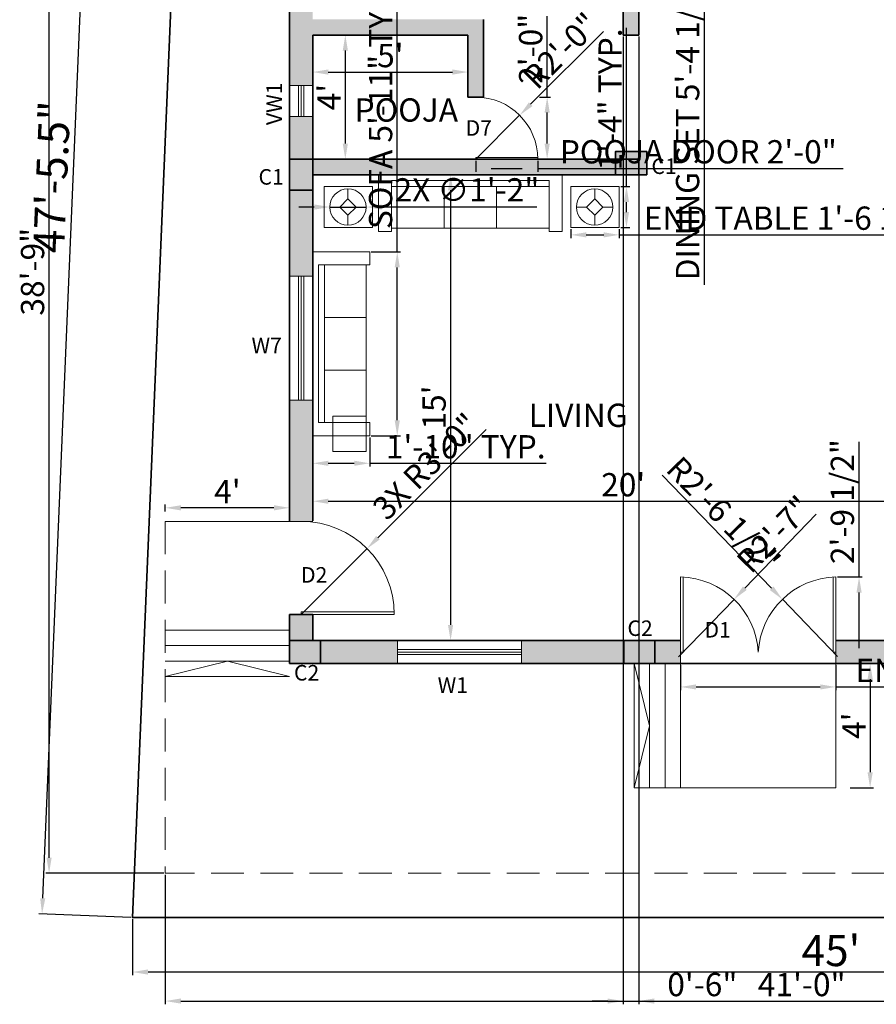
# Model space of a CAD drawing. Units: inches. Extents: x 4312 to 4955, y 6030 to 6717.
# Tile 1 of 5: x 4312 to 4643, y 6037 to 6418. Entities that reach past the tile are written whole.
import ezdxf

# ---------------------------------------------------------------- set-up
doc = ezdxf.new("R2010")
doc.units = ezdxf.units.IN
doc.linetypes.add('DASHED', pattern=[19.05, 12.7, -6.35])
for name, color, linetype, lineweight in [('A-AREA-IDEN', 7, 'Continuous', 20), ('A-FLOR-OVHD', 6, 'DASHED', 13), ('A-WALL', 7, 'Continuous', 35), ('C-PROP', 7, 'Continuous', 35), ('Dimensions', 112, 'Continuous', 13), ('Doors', 10, 'Continuous', 18), ('Furniture', 30, 'Continuous', 18), ('stair case', 130, 'Continuous', 18), ('Text', 30, 'Continuous', 18), ('Windows', 160, 'Continuous', 18)]:
    doc.layers.add(name, color=color, linetype=linetype, lineweight=lineweight)
doc.layers.add('A-WALL-PATT', color=251, linetype='Continuous', lineweight=13, true_color=0x636466)
doc.layers.add('Column', color=52, linetype='Continuous', lineweight=35, true_color=0xc8c92d)
doc.styles.get("Standard").update_dxf_attribs({"font": 'arial.ttf'})
doc.dimstyles.new('ISO-25', dxfattribs={"dimtxt": 9, "dimasz": 6, "dimexe": 1.25, "dimexo": 0.625, "dimtad": 1, "dimdec": 1, "dimlunit": 3, "dimtxsty": 'Standard', "dimcen": 2.5, "dimadec": 0, "dimazin": 0, "dimtfac": 1, "dimtdec": 1, "dimtmove": 0, "dimatfit": 3, "dimfxl": 1, "dimarcsym": 0})

# ---------------------------------------------------------------- blocks, each defined once
blk = doc.blocks.new('d1')
for p, q in [((4567.22, 6177.72), (4567.22, 6168.72)), ((4627.22, 6177.72), (4627.22, 6168.72))]:
    blk.add_line(p, q)
at = {"layer": 'Doors'}
for p, q in [((4567.22, 6173.22), (4567.22, 6202.22)), ((4568.22, 6173.22), (4568.22, 6202.22)), ((4626.22, 6173.22), (4626.22, 6202.22)), ((4627.22, 6173.22), (4627.22, 6202.22)), ((4567.22, 6173.22), (4568.22, 6173.22)), ((4626.22, 6173.22), (4627.22, 6173.22))]:
    blk.add_line(p, q, dxfattribs=at)
for centre, radius, start, end in [((4566.46, 6171.38), 30.85, 3.4285, 88.5806), ((4627.93, 6171.51), 30.72, 91.3248, 176.8002)]:
    blk.add_arc(centre, radius, start, end, dxfattribs=at)
blk = doc.blocks.new('d')
at = {"layer": 'Doors'}
for p, q in [((5019.4, 6368.39), (5043.4, 6368.39)), ((5019.4, 6367.72), (5019.4, 6368.39)), ((5019.4, 6367.72), (5043.4, 6367.72))]:
    blk.add_line(p, q, dxfattribs=at)
blk.add_arc((5019.4, 6367.72), 24, 0, 90, dxfattribs=at)
blk = doc.blocks.new('D2')
at = {"layer": 'Doors'}
for p, q in [((4718.9, 6093.56), (4754.9, 6093.56)), ((4718.9, 6092.56), (4718.9, 6093.56)), ((4718.9, 6092.56), (4754.9, 6092.56))]:
    blk.add_line(p, q, dxfattribs=at)
blk.add_arc((4718.9, 6092.56), 36, 0, 90, dxfattribs=at)
blk = doc.blocks.new('W')
at = {"layer": 'Windows'}
for p, q in [((4457.75, 6177.72), (4457.75, 6168.72)), ((4505.75, 6177.72), (4505.75, 6168.72)), ((4457.75, 6174.22), (4505.75, 6174.22)), ((4457.75, 6173.22), (4505.75, 6173.22)), ((4457.75, 6172.22), (4505.75, 6172.22))]:
    blk.add_line(p, q, dxfattribs=at)
blk = doc.blocks.new('*D21')
at = {"layer": 'Defpoints', "color": 0, "transparency": 16777216}
for p in [(4425.05, 6231.5), (4665.05, 6231.5), (4665.05, 6231.5)]:
    blk.add_point(p, dxfattribs=at)
at = {"layer": 'Dimensions', "color": 0, "lineweight": -2, "transparency": 16777216}
for p, q in [((4425.05, 6232.12), (4425.05, 6232.75)), ((4431.05, 6231.5), (4659.05, 6231.5)), ((4665.05, 6232.12), (4665.05, 6232.75))]:
    blk.add_line(p, q, dxfattribs=at)
at = {"layer": 'Dimensions', "color": 0, "transparency": 16777216}
for points in [[(4431.05, 6232.5), (4431.05, 6230.5), (4425.05, 6231.5)], [(4659.05, 6232.5), (4659.05, 6230.5), (4665.05, 6231.5)]]:
    blk.add_solid(points, dxfattribs=at)
at = {"layer": 'Dimensions', "color": 0, "transparency": 16777216, "insert": (4545.05, 6236.72), "char_height": 9, "attachment_point": 5}
blk.add_mtext("20'", dxfattribs=at)
blk = doc.blocks.new('*D22')
at = {"layer": 'Defpoints', "color": 0, "transparency": 16777216}
for p in [(4439.92, 6411.72), (4437.63, 6363.72), (4439.92, 6363.72)]:
    blk.add_point(p, dxfattribs=at)
at = {"layer": 'Dimensions', "color": 0, "lineweight": -2, "transparency": 16777216}
for p, q in [((4439.29, 6411.72), (4436.38, 6411.72)), ((4437.63, 6405.72), (4437.63, 6369.72)), ((4439.29, 6363.72), (4436.38, 6363.72))]:
    blk.add_line(p, q, dxfattribs=at)
at = {"layer": 'Dimensions', "color": 0, "transparency": 16777216}
for points in [[(4436.63, 6405.72), (4438.63, 6405.72), (4437.63, 6411.72)], [(4436.63, 6369.72), (4438.63, 6369.72), (4437.63, 6363.72)]]:
    blk.add_solid(points, dxfattribs=at)
at = {"layer": 'Dimensions', "color": 0, "transparency": 16777216, "insert": (4432.5, 6387.72), "char_height": 9, "attachment_point": 5, "rotation": 90}
blk.add_mtext("4'", dxfattribs=at)
blk = doc.blocks.new('*D23')
at = {"layer": 'Defpoints', "color": 0, "transparency": 16777216}
for p in [(4425.05, 6400.45), (4485.05, 6400.45), (4485.05, 6397.4)]:
    blk.add_point(p, dxfattribs=at)
at = {"layer": 'Dimensions', "color": 0, "lineweight": -2, "transparency": 16777216}
for p, q in [((4425.05, 6399.83), (4425.05, 6396.15)), ((4485.05, 6399.83), (4485.05, 6396.15)), ((4431.05, 6397.4), (4479.05, 6397.4))]:
    blk.add_line(p, q, dxfattribs=at)
at = {"layer": 'Dimensions', "color": 0, "transparency": 16777216}
for points in [[(4431.05, 6398.4), (4431.05, 6396.4), (4425.05, 6397.4)], [(4479.05, 6398.4), (4479.05, 6396.4), (4485.05, 6397.4)]]:
    blk.add_solid(points, dxfattribs=at)
at = {"layer": 'Dimensions', "color": 0, "transparency": 16777216, "insert": (4455.05, 6402.61), "char_height": 9, "attachment_point": 5}
blk.add_mtext("5'", dxfattribs=at)
blk = doc.blocks.new('*D24')
at = {"layer": 'Defpoints', "color": 0, "transparency": 16777216}
for p in [(4632.22, 6168.72), (4632.22, 6120.72), (4640.51, 6120.72)]:
    blk.add_point(p, dxfattribs=at)
at = {"layer": 'Dimensions', "color": 0, "lineweight": -2, "transparency": 16777216}
for p, q in [((4632.84, 6168.72), (4641.76, 6168.72)), ((4640.51, 6162.72), (4640.51, 6126.72)), ((4632.84, 6120.72), (4641.76, 6120.72))]:
    blk.add_line(p, q, dxfattribs=at)
at = {"layer": 'Dimensions', "color": 0, "transparency": 16777216}
for points in [[(4639.51, 6162.72), (4641.51, 6162.72), (4640.51, 6168.72)], [(4639.51, 6126.72), (4641.51, 6126.72), (4640.51, 6120.72)]]:
    blk.add_solid(points, dxfattribs=at)
at = {"layer": 'Dimensions', "color": 0, "transparency": 16777216, "insert": (4635.39, 6144.72), "char_height": 9, "attachment_point": 5, "rotation": 90}
blk.add_mtext("4'", dxfattribs=at)
blk = doc.blocks.new('*D26')
at = {"layer": 'Defpoints', "color": 0, "transparency": 16777216}
for p in [(4368.05, 6228.96), (4368.05, 6226.86), (4416.05, 6226.86)]:
    blk.add_point(p, dxfattribs=at)
at = {"layer": 'Dimensions', "color": 0, "lineweight": -2, "transparency": 16777216}
for p, q in [((4368.05, 6227.49), (4368.05, 6230.21)), ((4410.05, 6228.96), (4374.05, 6228.96)), ((4416.05, 6227.49), (4416.05, 6230.21))]:
    blk.add_line(p, q, dxfattribs=at)
at = {"layer": 'Dimensions', "color": 0, "transparency": 16777216}
for points in [[(4374.05, 6229.96), (4374.05, 6227.96), (4368.05, 6228.96)], [(4410.05, 6229.96), (4410.05, 6227.96), (4416.05, 6228.96)]]:
    blk.add_solid(points, dxfattribs=at)
at = {"layer": 'Dimensions', "color": 0, "transparency": 16777216, "insert": (4392.05, 6234.09), "char_height": 9, "attachment_point": 5}
blk.add_mtext("4'", dxfattribs=at)
blk = doc.blocks.new('*D37')
at = {"layer": 'Defpoints', "color": 0, "transparency": 16777216}
for p in [(4485.98, 6357.72), (4478.32, 6177.72), (4485.98, 6177.72)]:
    blk.add_point(p, dxfattribs=at)
at = {"layer": 'Dimensions', "color": 0, "lineweight": -2, "transparency": 16777216}
for p, q in [((4485.35, 6357.72), (4477.07, 6357.72)), ((4478.32, 6351.72), (4478.32, 6183.72)), ((4485.35, 6177.72), (4477.07, 6177.72))]:
    blk.add_line(p, q, dxfattribs=at)
at = {"layer": 'Dimensions', "color": 0, "transparency": 16777216}
for points in [[(4477.32, 6351.72), (4479.32, 6351.72), (4478.32, 6357.72)], [(4477.32, 6183.72), (4479.32, 6183.72), (4478.32, 6177.72)]]:
    blk.add_solid(points, dxfattribs=at)
at = {"layer": 'Dimensions', "color": 0, "transparency": 16777216, "insert": (4473.1, 6267.72), "char_height": 9, "attachment_point": 5, "rotation": 90}
blk.add_mtext("15'", dxfattribs=at)
blk = doc.blocks.new('*D42')
at = {"layer": 'Defpoints', "color": 0, "transparency": 16777216}
for p in [(4355.36, 6070.55), (4895.36, 6070.55), (4355.36, 6049.53)]:
    blk.add_point(p, dxfattribs=at)
at = {"layer": 'Dimensions', "color": 0, "lineweight": -2, "transparency": 16777216}
for p, q in [((4355.36, 6069.92), (4355.36, 6048.28)), ((4895.36, 6069.92), (4895.36, 6048.28)), ((4889.36, 6049.53), (4361.36, 6049.53))]:
    blk.add_line(p, q, dxfattribs=at)
at = {"layer": 'Dimensions', "color": 0, "transparency": 16777216}
for points in [[(4361.36, 6050.53), (4361.36, 6048.53), (4355.36, 6049.53)], [(4889.36, 6050.53), (4889.36, 6048.53), (4895.36, 6049.53)]]:
    blk.add_solid(points, dxfattribs=at)
at = {"layer": 'Dimensions', "color": 0, "transparency": 16777216, "insert": (4625.36, 6056.26), "char_height": 12, "attachment_point": 5}
blk.add_mtext("45'", dxfattribs=at)
blk = doc.blocks.new('*D43')
at = {"layer": 'Defpoints', "color": 0, "transparency": 16777216}
for p in [(4344.4, 6641.02), (4379.36, 6639.55), (4355.36, 6070.55)]:
    blk.add_point(p, dxfattribs=at)
at = {"layer": 'Dimensions', "color": 0, "lineweight": -2, "transparency": 16777216}
for p, q in [((4378.74, 6639.57), (4343.16, 6641.08)), ((4320.66, 6078.02), (4344.15, 6635.03)), ((4354.74, 6070.57), (4319.16, 6072.08))]:
    blk.add_line(p, q, dxfattribs=at)
at = {"layer": 'Dimensions', "color": 0, "transparency": 16777216}
for points in [[(4343.15, 6635.07), (4345.15, 6634.99), (4344.4, 6641.02)], [(4319.66, 6078.06), (4321.66, 6077.98), (4320.4, 6072.02)]]:
    blk.add_solid(points, dxfattribs=at)
at = {"layer": 'Dimensions', "color": 0, "transparency": 16777216, "insert": (4325.68, 6356.81), "char_height": 12, "attachment_point": 5, "rotation": 87.5847}
blk.add_mtext('47\'-5.5"', dxfattribs=at)
blk = doc.blocks.new('SOFA-THREE-SEAT')
for p, q in [((0, 71.06), (22, 71.06)), ((22, 71.06), (22, 65.99)), ((22, 65.99), (2.21, 65.99)), ((2.21, 5.08), (2.21, 65.99)), ((4.55, 5.08), (4.55, 65.99)), ((20.68, 5.08), (20.68, 65.99)), ((20.68, 45.68), (4.55, 45.68)), ((20.68, 25.38), (4.55, 25.38)), ((22, 5.08), (2.21, 5.08)), ((22, 5.08), (22, 0)), ((22, 0), (0, 0))]:
    blk.add_line(p, q)
blk = doc.blocks.new('END-TABLE-LAMP')
for p, q in [((9.23, 14.95), (9.23, 11.16)), ((2.23, 7.95), (6.03, 7.95)), ((16.23, 7.95), (12.43, 7.95)), ((9.23, 0.95), (9.23, 4.74))]:
    blk.add_line(p, q)
for points in [[(18.71, 15.9), (18.71, 0), (0, 0), (0, 15.9)], [(9.23, 11.16), (12.43, 7.95), (9.23, 4.74), (6.03, 7.95)]]:
    blk.add_lwpolyline(points, close=True)
blk.add_circle((9.23, 7.95), 7)
blk = doc.blocks.new('COLUMN-9X12-EDGE')
h = blk.add_hatch(color=256)
h.dxf.hatch_style = 1
h.paths.add_polyline_path([(9, 12), (0, 12), (0, 0), (9, 0)])
blk.add_lwpolyline([(9, 0), (0, 0)])
blk = doc.blocks.new('COLUMN-12X9-INLINE')
h = blk.add_hatch(color=256)
h.dxf.hatch_style = 1
h.paths.add_polyline_path([(12, 0), (12, 9), (0, 9), (0, 0)])
for points in [[(0, 0), (0, 9)], [(12, 9), (12, 0)]]:
    blk.add_lwpolyline(points)
blk = doc.blocks.new('*D67')
at = {"layer": 'Defpoints', "color": 0, "transparency": 16777216}
for p in [(4567.22, 6168.72), (4627.22, 6168.72), (4627.22, 6159.72)]:
    blk.add_point(p, dxfattribs=at)
at = {"layer": 'Dimensions', "color": 0, "lineweight": -2, "transparency": 16777216}
for p, q in [((4567.22, 6168.1), (4567.22, 6158.47)), ((4627.22, 6168.1), (4627.22, 6158.47)), ((4573.22, 6159.72), (4621.22, 6159.72)), ((4627.22, 6159.72), (4704.03, 6159.72))]:
    blk.add_line(p, q, dxfattribs=at)
at = {"layer": 'Dimensions', "color": 0, "transparency": 16777216}
for points in [[(4573.22, 6160.72), (4573.22, 6158.72), (4567.22, 6159.72)], [(4621.22, 6160.72), (4621.22, 6158.72), (4627.22, 6159.72)]]:
    blk.add_solid(points, dxfattribs=at)
at = {"layer": 'Dimensions', "color": 0, "transparency": 16777216, "insert": (4668.63, 6164.94), "char_height": 9, "attachment_point": 5}
blk.add_mtext('ENTRY 5\'-0"', dxfattribs=at)
blk = doc.blocks.new('*D68')
at = {"layer": 'Defpoints', "color": 0, "transparency": 16777216}
for p in [(4627.22, 6202.22), (4636.22, 6202.22), (4627.22, 6168.72)]:
    blk.add_point(p, dxfattribs=at)
at = {"layer": 'Dimensions', "color": 0, "lineweight": -2, "transparency": 16777216}
for p, q in [((4636.22, 6202.22), (4636.22, 6254.52)), ((4627.85, 6202.22), (4637.47, 6202.22)), ((4636.22, 6174.72), (4636.22, 6196.22)), ((4627.85, 6168.72), (4637.47, 6168.72))]:
    blk.add_line(p, q, dxfattribs=at)
at = {"layer": 'Dimensions', "color": 0, "transparency": 16777216}
for points in [[(4635.22, 6196.22), (4637.22, 6196.22), (4636.22, 6202.22)], [(4635.22, 6174.72), (4637.22, 6174.72), (4636.22, 6168.72)]]:
    blk.add_solid(points, dxfattribs=at)
at = {"layer": 'Dimensions', "color": 0, "transparency": 16777216, "insert": (4630.94, 6231.37), "char_height": 9, "attachment_point": 5, "rotation": 90}
blk.add_mtext('2\'-9 1/2"', dxfattribs=at)
blk = doc.blocks.new('*D69')
at = {"layer": 'Defpoints', "color": 0, "transparency": 16777216}
for p in [(4488.05, 6363.72), (4512.05, 6363.72), (4512.05, 6360.12)]:
    blk.add_point(p, dxfattribs=at)
at = {"layer": 'Dimensions', "color": 0, "lineweight": -2, "transparency": 16777216}
for p, q in [((4488.05, 6363.1), (4488.05, 6358.87)), ((4494.05, 6360.12), (4506.05, 6360.12)), ((4512.05, 6363.1), (4512.05, 6358.87)), ((4512.05, 6360.12), (4630.1, 6360.12))]:
    blk.add_line(p, q, dxfattribs=at)
at = {"layer": 'Dimensions', "color": 0, "transparency": 16777216}
for points in [[(4494.05, 6361.12), (4494.05, 6359.12), (4488.05, 6360.12)], [(4506.05, 6361.12), (4506.05, 6359.12), (4512.05, 6360.12)]]:
    blk.add_solid(points, dxfattribs=at)
at = {"layer": 'Dimensions', "color": 0, "transparency": 16777216, "insert": (4574.07, 6365.41), "char_height": 9, "attachment_point": 5}
blk.add_mtext('POOJA DOOR 2\'-0"', dxfattribs=at)
blk = doc.blocks.new('*D70')
at = {"layer": 'Defpoints', "color": 0, "transparency": 16777216}
for p in [(4512.05, 6387.72), (4515.65, 6387.72), (4512.05, 6363.72)]:
    blk.add_point(p, dxfattribs=at)
at = {"layer": 'Dimensions', "color": 0, "lineweight": -2, "transparency": 16777216}
for p, q in [((4515.65, 6387.72), (4515.65, 6419.05)), ((4512.67, 6387.72), (4516.9, 6387.72)), ((4515.65, 6369.72), (4515.65, 6381.72)), ((4512.67, 6363.72), (4516.9, 6363.72))]:
    blk.add_line(p, q, dxfattribs=at)
at = {"layer": 'Dimensions', "color": 0, "transparency": 16777216}
for points in [[(4514.65, 6381.72), (4516.65, 6381.72), (4515.65, 6387.72)], [(4514.65, 6369.72), (4516.65, 6369.72), (4515.65, 6363.72)]]:
    blk.add_solid(points, dxfattribs=at)
at = {"layer": 'Dimensions', "color": 0, "transparency": 16777216, "insert": (4510.43, 6406.39), "char_height": 9, "attachment_point": 5, "rotation": 90}
blk.add_mtext('2\'-0"', dxfattribs=at)
blk = doc.blocks.new('*D73')
at = {"layer": 'Defpoints', "color": 0, "transparency": 16777216}
for p in [(4447.05, 6327.89), (4457.7, 6327.89), (4447.05, 6256.83)]:
    blk.add_point(p, dxfattribs=at)
at = {"layer": 'Dimensions', "color": 0, "lineweight": -2, "transparency": 16777216}
for p, q in [((4457.7, 6327.89), (4457.7, 6434.68)), ((4447.67, 6327.89), (4458.95, 6327.89)), ((4457.7, 6262.83), (4457.7, 6321.89)), ((4447.67, 6256.83), (4458.95, 6256.83))]:
    blk.add_line(p, q, dxfattribs=at)
at = {"layer": 'Dimensions', "color": 0, "transparency": 16777216}
for points in [[(4456.7, 6321.89), (4458.7, 6321.89), (4457.7, 6327.89)], [(4456.7, 6262.83), (4458.7, 6262.83), (4457.7, 6256.83)]]:
    blk.add_solid(points, dxfattribs=at)
at = {"layer": 'Dimensions', "color": 0, "transparency": 16777216, "insert": (4452.42, 6384.28), "char_height": 9, "attachment_point": 5, "rotation": 90}
blk.add_mtext('SOFA 5\'-11" TYP.', dxfattribs=at)
blk = doc.blocks.new('*D74')
at = {"layer": 'Defpoints', "color": 0, "transparency": 16777216}
for p in [(4425.05, 6256.83), (4447.05, 6256.83), (4447.05, 6246.17)]:
    blk.add_point(p, dxfattribs=at)
at = {"layer": 'Dimensions', "color": 0, "lineweight": -2, "transparency": 16777216}
for p, q in [((4425.05, 6256.2), (4425.05, 6244.92)), ((4447.05, 6256.2), (4447.05, 6244.92)), ((4431.05, 6246.17), (4441.05, 6246.17)), ((4447.05, 6246.17), (4515.3, 6246.17))]:
    blk.add_line(p, q, dxfattribs=at)
at = {"layer": 'Dimensions', "color": 0, "transparency": 16777216}
for points in [[(4431.05, 6247.17), (4431.05, 6245.17), (4425.05, 6246.17)], [(4441.05, 6247.17), (4441.05, 6245.17), (4447.05, 6246.17)]]:
    blk.add_solid(points, dxfattribs=at)
at = {"layer": 'Dimensions', "color": 0, "transparency": 16777216, "insert": (4484.17, 6251.39), "char_height": 9, "attachment_point": 5}
blk.add_mtext('1\'-10" TYP.', dxfattribs=at)
blk = doc.blocks.new('*D75')
at = {"layer": 'Defpoints', "color": 0, "transparency": 16777216}
for p in [(4524.79, 6337.28), (4543.5, 6337.28), (4543.5, 6334.47)]:
    blk.add_point(p, dxfattribs=at)
at = {"layer": 'Dimensions', "color": 0, "lineweight": -2, "transparency": 16777216}
for p, q in [((4524.79, 6336.65), (4524.79, 6333.22)), ((4530.79, 6334.47), (4537.5, 6334.47)), ((4543.5, 6336.65), (4543.5, 6333.22)), ((4543.5, 6334.47), (4699.47, 6334.47))]:
    blk.add_line(p, q, dxfattribs=at)
at = {"layer": 'Dimensions', "color": 0, "transparency": 16777216}
for points in [[(4530.79, 6335.47), (4530.79, 6333.47), (4524.79, 6334.47)], [(4537.5, 6335.47), (4537.5, 6333.47), (4543.5, 6334.47)]]:
    blk.add_solid(points, dxfattribs=at)
at = {"layer": 'Dimensions', "color": 0, "transparency": 16777216, "insert": (4624.48, 6339.75), "char_height": 9, "attachment_point": 5}
blk.add_mtext('END TABLE 1\'-6 1/2" TYP.', dxfattribs=at)
blk = doc.blocks.new('*D76')
at = {"layer": 'Defpoints', "color": 0, "transparency": 16777216}
for p in [(4543.5, 6353.17), (4546.31, 6353.17), (4543.5, 6337.28)]:
    blk.add_point(p, dxfattribs=at)
at = {"layer": 'Dimensions', "color": 0, "lineweight": -2, "transparency": 16777216}
for p, q in [((4546.31, 6353.17), (4546.31, 6414.43)), ((4544.12, 6353.17), (4547.56, 6353.17)), ((4546.31, 6343.28), (4546.31, 6347.17)), ((4544.12, 6337.28), (4547.56, 6337.28))]:
    blk.add_line(p, q, dxfattribs=at)
at = {"layer": 'Dimensions', "color": 0, "transparency": 16777216}
for points in [[(4545.31, 6347.17), (4547.31, 6347.17), (4546.31, 6353.17)], [(4545.31, 6343.28), (4547.31, 6343.28), (4546.31, 6337.28)]]:
    blk.add_solid(points, dxfattribs=at)
at = {"layer": 'Dimensions', "color": 0, "transparency": 16777216, "insert": (4541.16, 6386.8), "char_height": 9, "attachment_point": 5, "rotation": 90}
blk.add_mtext('1\'-4" TYP.', dxfattribs=at)
blk = doc.blocks.new('*D83')
at = {"layer": 'Defpoints', "color": 0, "transparency": 16777216}
for p in [(4586.05, 6506.69), (4576.38, 6442.24), (4586.05, 6442.24)]:
    blk.add_point(p, dxfattribs=at)
at = {"layer": 'Dimensions', "color": 0, "lineweight": -2, "transparency": 16777216}
for p, q in [((4585.42, 6506.69), (4575.13, 6506.69)), ((4576.38, 6500.69), (4576.38, 6448.24)), ((4585.42, 6442.24), (4575.13, 6442.24)), ((4576.38, 6442.24), (4576.38, 6315.1))]:
    blk.add_line(p, q, dxfattribs=at)
at = {"layer": 'Dimensions', "color": 0, "transparency": 16777216}
for points in [[(4575.38, 6500.69), (4577.38, 6500.69), (4576.38, 6506.69)], [(4575.38, 6448.24), (4577.38, 6448.24), (4576.38, 6442.24)]]:
    blk.add_solid(points, dxfattribs=at)
at = {"layer": 'Dimensions', "color": 0, "transparency": 16777216, "insert": (4571.1, 6375.67), "char_height": 9, "attachment_point": 5, "rotation": 90}
blk.add_mtext('DINING SET 5\'-4 1/2"', dxfattribs=at)
blk = doc.blocks.new('*D89')
at = {"layer": 'Defpoints', "color": 0, "transparency": 16777216}
for p in [(4860.05, 6090.72), (4368.05, 6087.72), (4860.05, 6038.3)]:
    blk.add_point(p, dxfattribs=at)
at = {"layer": 'Dimensions', "color": 0, "lineweight": -2, "transparency": 16777216}
for p, q in [((4860.05, 6090.1), (4860.05, 6037.05)), ((4368.05, 6087.1), (4368.05, 6037.05)), ((4374.05, 6038.3), (4854.05, 6038.3))]:
    blk.add_line(p, q, dxfattribs=at)
at = {"layer": 'Dimensions', "color": 0, "transparency": 16777216}
for points in [[(4374.05, 6039.3), (4374.05, 6037.3), (4368.05, 6038.3)], [(4854.05, 6039.3), (4854.05, 6037.3), (4860.05, 6038.3)]]:
    blk.add_solid(points, dxfattribs=at)
at = {"layer": 'Dimensions', "color": 0, "transparency": 16777216, "insert": (4614.05, 6043.52), "char_height": 9, "attachment_point": 5}
blk.add_mtext('41\'-0"', dxfattribs=at)
blk = doc.blocks.new('*D90')
at = {"layer": 'Defpoints', "color": 0, "transparency": 16777216}
for p in [(4323.11, 6552.72), (4416.05, 6552.72), (4368.05, 6087.72)]:
    blk.add_point(p, dxfattribs=at)
at = {"layer": 'Dimensions', "color": 0, "lineweight": -2, "transparency": 16777216}
for p, q in [((4415.42, 6552.72), (4321.86, 6552.72)), ((4323.11, 6093.72), (4323.11, 6546.72)), ((4367.42, 6087.72), (4321.86, 6087.72))]:
    blk.add_line(p, q, dxfattribs=at)
at = {"layer": 'Dimensions', "color": 0, "transparency": 16777216}
for points in [[(4322.11, 6546.72), (4324.11, 6546.72), (4323.11, 6552.72)], [(4322.11, 6093.72), (4324.11, 6093.72), (4323.11, 6087.72)]]:
    blk.add_solid(points, dxfattribs=at)
at = {"layer": 'Dimensions', "color": 0, "transparency": 16777216, "insert": (4317.89, 6320.22), "char_height": 9, "attachment_point": 5, "rotation": 90}
blk.add_mtext('38\'-9"', dxfattribs=at)
blk = doc.blocks.new('*D91')
at = {"layer": 'Defpoints', "color": 0, "transparency": 16777216}
for p in [(4545.05, 6411.72), (4551.05, 6411.72), (4551.05, 6038.3)]:
    blk.add_point(p, dxfattribs=at)
at = {"layer": 'Dimensions', "color": 0, "lineweight": -2, "transparency": 16777216}
for p, q in [((4545.05, 6411.1), (4545.05, 6037.05)), ((4551.05, 6411.1), (4551.05, 6037.05)), ((4539.05, 6038.3), (4533.05, 6038.3)), ((4545.05, 6038.3), (4551.05, 6038.3)), ((4557.05, 6038.3), (4588.22, 6038.3))]:
    blk.add_line(p, q, dxfattribs=at)
at = {"layer": 'Dimensions', "color": 0, "transparency": 16777216}
for points in [[(4539.05, 6039.3), (4539.05, 6037.3), (4545.05, 6038.3)], [(4557.05, 6039.3), (4557.05, 6037.3), (4551.05, 6038.3)]]:
    blk.add_solid(points, dxfattribs=at)
at = {"layer": 'Dimensions', "color": 0, "transparency": 16777216, "insert": (4575.64, 6043.52), "char_height": 9, "attachment_point": 5}
blk.add_mtext('0\'-6"', dxfattribs=at)
blk = doc.blocks.new('*D92')
at = {"layer": 'Defpoints', "color": 0, "transparency": 16777216}
for p in [(4431.65, 6345.22), (4445.65, 6345.22)]:
    blk.add_point(p, dxfattribs=at)
at = {"layer": 'Dimensions', "color": 0, "lineweight": -2, "transparency": 16777216}
for p, q in [((4425.65, 6345.22), (4419.65, 6345.22)), ((4431.65, 6345.22), (4445.65, 6345.22)), ((4511.63, 6345.23), (4451.65, 6345.22))]:
    blk.add_line(p, q, dxfattribs=at)
at = {"layer": 'Dimensions', "color": 0, "transparency": 16777216}
for points in [[(4425.65, 6346.22), (4425.65, 6344.22), (4431.65, 6345.22)], [(4451.65, 6346.22), (4451.65, 6344.22), (4445.65, 6345.22)]]:
    blk.add_solid(points, dxfattribs=at)
at = {"layer": 'Dimensions', "color": 0, "transparency": 16777216, "insert": (4484.64, 6350.7), "char_height": 9, "attachment_point": 5, "rotation": 0.0023}
blk.add_mtext('2X ∅1\'-2"', dxfattribs=at)
blk = doc.blocks.new('*D93')
at = {"layer": 'Defpoints', "color": 0, "transparency": 16777216}
for p in [(4587.89, 6193.58), (4566.46, 6171.38)]:
    blk.add_point(p, dxfattribs=at)
at = {"layer": 'Dimensions', "color": 0, "lineweight": -2, "transparency": 16777216}
for p, q in [((4619.69, 6226.52), (4592.06, 6197.89)), ((4566.46, 6171.38), (4587.89, 6193.58))]:
    blk.add_line(p, q, dxfattribs=at)
at = {"layer": 'Dimensions', "color": 0, "transparency": 16777216}
blk.add_solid([(4591.34, 6198.59), (4592.78, 6197.2), (4587.89, 6193.58)], dxfattribs=at)
at = {"layer": 'Dimensions', "color": 0, "transparency": 16777216, "insert": (4604.26, 6217.93), "char_height": 9, "attachment_point": 5, "rotation": 46.0044}
blk.add_mtext('R2\'-7"', dxfattribs=at)
blk = doc.blocks.new('*D94')
at = {"layer": 'Defpoints', "color": 0, "transparency": 16777216}
for p in [(4606.57, 6193.59), (4627.93, 6171.51)]:
    blk.add_point(p, dxfattribs=at)
at = {"layer": 'Dimensions', "color": 0, "lineweight": -2, "transparency": 16777216}
for p, q in [((4560.14, 6241.56), (4602.39, 6197.9)), ((4627.93, 6171.51), (4606.57, 6193.59))]:
    blk.add_line(p, q, dxfattribs=at)
at = {"layer": 'Dimensions', "color": 0, "transparency": 16777216}
blk.add_solid([(4603.11, 6198.59), (4601.68, 6197.2), (4606.57, 6193.59)], dxfattribs=at)
at = {"layer": 'Dimensions', "color": 0, "transparency": 16777216, "insert": (4582.97, 6225.56), "char_height": 9, "attachment_point": 5, "rotation": 314.0614}
blk.add_mtext('R2\'-6 1/2"', dxfattribs=at)
blk = doc.blocks.new('*D95')
at = {"layer": 'Defpoints', "color": 0, "transparency": 16777216}
for p in [(4446.01, 6213.18), (4420.55, 6187.72)]:
    blk.add_point(p, dxfattribs=at)
at = {"layer": 'Dimensions', "color": 0, "lineweight": -2, "transparency": 16777216}
for p, q in [((4492.05, 6259.23), (4450.25, 6217.42)), ((4420.55, 6187.72), (4446.01, 6213.18))]:
    blk.add_line(p, q, dxfattribs=at)
at = {"layer": 'Dimensions', "color": 0, "transparency": 16777216}
blk.add_solid([(4449.54, 6218.13), (4450.95, 6216.72), (4446.01, 6213.18)], dxfattribs=at)
at = {"layer": 'Dimensions', "color": 0, "transparency": 16777216, "insert": (4469.58, 6244.14), "char_height": 9, "attachment_point": 5, "rotation": 44.9999}
blk.add_mtext('3X R3\'-0"', dxfattribs=at)
blk = doc.blocks.new('*D97')
at = {"layer": 'Defpoints', "color": 0, "transparency": 16777216}
for p in [(4505.02, 6380.69), (4488.05, 6363.72)]:
    blk.add_point(p, dxfattribs=at)
at = {"layer": 'Dimensions', "color": 0, "lineweight": -2, "transparency": 16777216}
for p, q in [((4537.4, 6413.07), (4509.26, 6384.94)), ((4488.05, 6363.72), (4505.02, 6380.69))]:
    blk.add_line(p, q, dxfattribs=at)
at = {"layer": 'Dimensions', "color": 0, "transparency": 16777216}
blk.add_solid([(4508.56, 6385.64), (4509.97, 6384.23), (4505.02, 6380.69)], dxfattribs=at)
at = {"layer": 'Dimensions', "color": 0, "transparency": 16777216, "insert": (4521.76, 6404.82), "char_height": 9, "attachment_point": 5, "rotation": 44.9998}
blk.add_mtext('R2\'-0"', dxfattribs=at)

msp = doc.modelspace()

# ---------------------------------------------------------------- hatches: boundary and pattern name
at = {"layer": 'A-WALL-PATT'}
h = msp.add_hatch(color=256, dxfattribs=at)
h.dxf.hatch_style = 1
h.paths.add_polyline_path([(4551.05, 6540.72), (4545.05, 6540.72), (4545.05, 6411.72), (4551.05, 6411.72)])
h = msp.add_hatch(color=256, dxfattribs=at)
h.dxf.hatch_style = 1
h.paths.add_polyline_path([(4425.05, 6466.16), (4416.05, 6466.16), (4416.05, 6392.17), (4425.05, 6392.17), (4425.05, 6411.72), (4485.05, 6411.72), (4485.05, 6387.72), (4491.05, 6387.72), (4491.05, 6417.72), (4425.05, 6417.72)])
h = msp.add_hatch(color=256, dxfattribs=at)
h.dxf.hatch_style = 1
h.paths.add_polyline_path([(4425.05, 6380.17), (4416.05, 6380.17), (4416.05, 6363.72), (4425.05, 6363.72), (4425.05, 6357.72), (4542.13, 6357.72), (4542.13, 6363.72), (4425.05, 6363.72)])
h = msp.add_hatch(color=256, dxfattribs=at)
h.dxf.hatch_style = 1
h.paths.add_polyline_path([(4425.05, 6351.72), (4416.05, 6351.72), (4416.05, 6318.5), (4425.05, 6318.5)])
h = msp.add_hatch(color=256, dxfattribs=at)
h.dxf.hatch_style = 1
h.paths.add_polyline_path([(4425.05, 6270.53), (4416.05, 6270.53), (4416.05, 6223.72), (4425.05, 6223.72)])
h = msp.add_hatch(color=256, dxfattribs=at)
h.dxf.hatch_style = 1
h.paths.add_polyline_path([(4425.05, 6187.72), (4420.55, 6187.72), (4416.05, 6187.72), (4416.05, 6177.72), (4425.05, 6177.72)])
h = msp.add_hatch(color=256, dxfattribs=at)
h.dxf.hatch_style = 1
h.paths.add_polyline_path([(4457.75, 6177.72), (4428.05, 6177.72), (4428.05, 6168.72), (4457.75, 6168.72)])
h = msp.add_hatch(color=256, dxfattribs=at)
h.dxf.hatch_style = 1
h.paths.add_polyline_path([(4545.33, 6177.72), (4505.75, 6177.72), (4505.75, 6168.72), (4545.33, 6168.72)])
h = msp.add_hatch(color=256, dxfattribs=at)
h.dxf.hatch_style = 1
h.paths.add_polyline_path([(4567.22, 6177.72), (4557.33, 6177.72), (4557.33, 6168.72), (4567.22, 6168.72)])
h = msp.add_hatch(color=256, dxfattribs=at)
h.dxf.hatch_style = 1
h.paths.add_polyline_path([(4662.02, 6177.72), (4627.22, 6177.72), (4627.22, 6168.72), (4662.02, 6168.72)])
at = {"layer": 'Column'}
h = msp.add_hatch(color=256, dxfattribs=at)
h.dxf.hatch_style = 1
h.paths.add_polyline_path([(4554.13, 6357.72), (4554.13, 6366.72), (4542.13, 6366.72), (4542.13, 6357.72)])
h = msp.add_hatch(color=256, dxfattribs=at)
h.dxf.hatch_style = 1
h.paths.add_polyline_path([(4428.05, 6168.72), (4428.05, 6177.72), (4416.05, 6177.72), (4416.05, 6168.72)])

# ---------------------------------------------------------------- linework, layer by layer
at = {"layer": 'A-FLOR-OVHD'}
for p in [(4368.05, 6223.72), (4703.23, 6087.72)]:
    msp.add_line(p, (4368.05, 6087.72), dxfattribs=at)
at = {"layer": 'A-WALL'}
for p, q in [((4416.05, 6223.72), (4416.05, 6552.72)), ((4545.05, 6552.72), (4545.05, 6411.72)), ((4551.05, 6543.72), (4551.05, 6411.72)), ((4491.05, 6387.72), (4491.05, 6417.72)), ((4425.05, 6411.72), (4485.05, 6411.72)), ((4425.05, 6363.72), (4425.05, 6411.72)), ((4425.05, 6223.87), (4425.05, 6411.72)), ((4485.05, 6387.72), (4485.05, 6411.72)), ((4545.05, 6411.72), (4551.05, 6411.72)), ((4485.05, 6387.72), (4491.05, 6387.72)), ((4425.05, 6363.72), (4551.05, 6363.72)), ((4551.05, 6363.72), (4551.05, 6357.72)), ((4425.05, 6357.72), (4554.13, 6357.72)), ((4425.05, 6187.72), (4416.05, 6187.72)), ((4416.05, 6187.72), (4416.05, 6177.72)), ((4425.05, 6177.72), (4425.05, 6187.72)), ((4567.22, 6177.72), (4425.05, 6177.72)), ((4797.05, 6177.72), (4627.22, 6177.72)), ((4860.05, 6168.72), (4416.05, 6168.72)), ((4860.05, 6168.72), (4627.22, 6168.72))]:
    msp.add_line(p, q, dxfattribs=at)
for points in [[(4416.05, 6363.72), (4542.13, 6363.72)], [(4416.05, 6177.72), (4567.22, 6177.72)]]:
    msp.add_lwpolyline(points, dxfattribs=at)
at = {"layer": 'C-PROP'}
msp.add_lwpolyline([(4895.36, 6639.55), (4895.36, 6070.55), (4355.36, 6070.55), (4379.36, 6639.55)], close=True, dxfattribs=at)
at = {"layer": 'Column'}
msp.add_line((4416.05, 6177.72), (4416.05, 6168.72), dxfattribs=at)
for points in [[(4542.13, 6357.72), (4542.13, 6366.72), (4554.13, 6366.72), (4554.13, 6357.72)], [(4428.05, 6177.72), (4428.05, 6168.72)]]:
    msp.add_lwpolyline(points, dxfattribs=at)
at = {"layer": 'Furniture'}
for p, q in [((4432.74, 6264.45), (4432.74, 6250.77)), ((4445.73, 6264.45), (4432.74, 6264.45)), ((4445.73, 6250.77), (4445.73, 6264.45)), ((4432.74, 6250.77), (4445.73, 6250.77))]:
    msp.add_line(p, q, dxfattribs=at)
at = {"layer": 'stair case'}
for p, q in [((4368.05, 6223.72), (4425.05, 6223.72)), ((4416.05, 6181.72), (4368.05, 6181.72)), ((4416.05, 6175.72), (4368.05, 6175.72)), ((4416.05, 6169.72), (4368.05, 6169.72)), ((4368.05, 6163.72), (4392.05, 6169.72)), ((4392.05, 6169.72), (4416.05, 6163.72)), ((4549.22, 6168.72), (4549.22, 6120.72)), ((4549.22, 6168.72), (4555.22, 6144.72)), ((4555.22, 6168.72), (4555.22, 6120.72)), ((4561.22, 6168.72), (4561.22, 6120.72)), ((4567.22, 6168.72), (4567.22, 6120.72)), ((4627.22, 6168.72), (4627.22, 6120.72)), ((4416.05, 6163.72), (4368.05, 6163.72)), ((4555.22, 6144.72), (4549.22, 6120.72)), ((4627.22, 6120.72), (4549.22, 6120.72))]:
    msp.add_line(p, q, dxfattribs=at)
at = {"layer": 'Windows'}
for p, q in [((4425.05, 6392.17), (4416.05, 6392.17)), ((4419.55, 6392.17), (4419.55, 6380.17)), ((4420.55, 6392.17), (4420.55, 6380.17)), ((4421.55, 6392.17), (4421.55, 6380.17)), ((4425.05, 6380.17), (4416.05, 6380.17)), ((4425.05, 6318.5), (4416.05, 6318.5)), ((4419.55, 6318.53), (4419.55, 6270.53)), ((4420.55, 6318.53), (4420.55, 6270.53)), ((4421.55, 6318.53), (4421.55, 6270.53)), ((4425.05, 6270.53), (4416.05, 6270.53))]:
    msp.add_line(p, q, dxfattribs=at)

# ---------------------------------------------------------------- block references
at = {"layer": 'Column', "rotation": 359.9985405731541}
msp.add_blockref('COLUMN-9X12-EDGE', (4416.05, 6351.72), dxfattribs=at)
at = {"layer": 'Column'}
msp.add_blockref('COLUMN-12X9-INLINE', (4545.33, 6168.72), dxfattribs=at)
at = {"layer": 'Doors'}
for name, p in [('d', (-531.35, -4)), ('D2', (-298.35, 95.16)), ('d1', (0, 0))]:
    msp.add_blockref(name, p, dxfattribs=at)
at = {"layer": 'Furniture', "rotation": 269.9999999999987}
msp.add_blockref('SOFA-THREE-SEAT', (4450.44, 6357.72), dxfattribs=at)
at = {"layer": 'Furniture'}
for name, p in [('END-TABLE-LAMP', (4429.42, 6337.28)), ('END-TABLE-LAMP', (4524.79, 6337.28)), ('SOFA-THREE-SEAT', (4425.05, 6256.83))]:
    msp.add_blockref(name, p, dxfattribs=at)
at = {"layer": 'Windows'}
msp.add_blockref('W', (0, 0), dxfattribs=at)

# ---------------------------------------------------------------- texts
at = {"layer": 'A-AREA-IDEN', "char_height": 9, "attachment_point": 1, "rotation": 0.0025}
for s, insert in [('POOJA', (4441.19, 6387.23)), ('LIVING', (4508.5, 6269.23))]:
    msp.add_mtext_dynamic_manual_height_columns(s, width=10.4718, gutter_width=12.5, heights=[0], dxfattribs=dict(at, insert=insert))
at = {"layer": 'Text', "insert": (4407.14, 6376.9), "char_height": 6, "attachment_point": 1, "rotation": 90}
msp.add_mtext_dynamic_manual_height_columns('VW1', width=19.9533, gutter_width=12.5, heights=[0], dxfattribs=at)
at = {"layer": 'Text', "char_height": 6, "attachment_point": 1}
for s, insert in [('D7', (4484.13, 6378.79)), ('C1', (4555.96, 6363.99)), ('C1', (4404.08, 6359.88)), ('W7', (4401.37, 6294.73)), ('D2', (4420.5, 6206.04)), ('C2', (4546.68, 6185.43)), ('D1', (4576.48, 6184.82)), ('C2', (4417.78, 6168.2)), ('W1', (4473.32, 6163.42))]:
    msp.add_mtext_dynamic_manual_height_columns(s, width=4.4911, gutter_width=12.5, heights=[0], dxfattribs=dict(at, insert=insert))

# ---------------------------------------------------------------- dimensions: what is measured, and where the dimension line sits
at = {"layer": 'Dimensions'}
dim = msp.add_aligned_dim(p1=(4355.36, 6070.55), p2=(4379.36, 6639.55), distance=34.99, dimstyle='ISO-25', override={"dimtxt": 12, "dimclrd": 0, "dimclre": 0, "dimclrt": 0}, dxfattribs=at)
dim.commit()
dim.dimension.update_dxf_attribs({"geometry": '*D43', "text_midpoint": (4325.68, 6356.81)})
for base, p1, p2, override, picture, middle in [((4323.11, 6552.72), (4368.05, 6087.72), (4416.05, 6552.72), {"dimdec": 1, "dimlfac": 1, "dimrnd": 0, "dimzin": 1, "dimdsep": 46, "dimlunit": 4, "dimfrac": 2}, '*D90', (4317.89, 6320.22)), ((4515.65, 6387.72), (4512.05, 6363.72), (4512.05, 6387.72), {"dimdec": 1, "dimlfac": 1, "dimrnd": 0, "dimzin": 1, "dimdsep": 46, "dimlunit": 4, "dimfrac": 2}, '*D70', (4510.43, 6406.39)), ((4437.63, 6363.72), (4439.92, 6411.72), (4439.92, 6363.72), {"dimclrd": 0, "dimclre": 0, "dimclrt": 0}, '*D22', (4432.5, 6387.72)), ((4478.32, 6177.72), (4485.98, 6357.72), (4485.98, 6177.72), {"dimclrd": 0, "dimclre": 0, "dimclrt": 0}, '*D37', (4473.1, 6267.72)), ((4636.22, 6202.22), (4627.22, 6168.72), (4627.22, 6202.22), {"dimdec": 1, "dimlfac": 1, "dimrnd": 0, "dimzin": 1, "dimdsep": 46, "dimlunit": 4, "dimfrac": 2}, '*D68', (4630.94, 6231.37)), ((4640.51, 6120.72), (4632.22, 6168.72), (4632.22, 6120.72), {"dimclrd": 0, "dimclre": 0, "dimclrt": 0}, '*D24', (4635.39, 6144.72))]:
    dim = msp.add_linear_dim(base=base, p1=p1, p2=p2, angle=90, dimstyle='ISO-25', override=override, dxfattribs=at)
    dim.commit()
    dim.dimension.update_dxf_attribs({"geometry": picture, "text_midpoint": middle})
for base, p1, p2, angle, text, picture, middle in [((4576.3781, 6442.2371), (4586.0462, 6506.6912), (4586.0462, 6442.2371), 270, 'DINING SET <>', '*D83', (4571.0996, 6375.6663)), ((4457.7, 6327.89), (4447.05, 6256.83), (4447.05, 6327.89), 90, 'SOFA <> TYP.', '*D73', (4452.42, 6384.28)), ((4546.31, 6353.17), (4543.5, 6337.28), (4543.5, 6353.17), 90, '<> TYP.', '*D76', (4541.16, 6386.8))]:
    dim = msp.add_linear_dim(base=base, p1=p1, p2=p2, angle=angle, text=text, dimstyle='ISO-25', override={"dimdec": 1, "dimlfac": 1, "dimrnd": 0, "dimzin": 1, "dimdsep": 46, "dimlunit": 4, "dimfrac": 2}, dxfattribs=at)
    dim.commit()
    dim.dimension.update_dxf_attribs({"geometry": picture, "text_midpoint": middle})
for center, mpoint, picture, middle in [((4488.05, 6363.72), (4505.02, 6380.69), '*D97', (4521.76, 6404.82)), ((4627.93, 6171.51), (4606.57, 6193.59), '*D94', (4582.97, 6225.56)), ((4566.46, 6171.38), (4587.89, 6193.58), '*D93', (4604.26, 6217.93))]:
    dim = msp.add_radius_dim(center=center, mpoint=mpoint, dimstyle='ISO-25', override={"dimdec": 1, "dimlfac": 1, "dimrnd": 0, "dimzin": 1, "dimdsep": 46, "dimlunit": 4, "dimfrac": 2}, dxfattribs=at)
    dim.commit()
    dim.dimension.update_dxf_attribs({"geometry": picture, "text_midpoint": middle})
for base, p1, p2, override, picture, middle in [((4551.05, 6038.3), (4545.05, 6411.72), (4551.05, 6411.72), {"dimdec": 1, "dimlfac": 1, "dimrnd": 0, "dimzin": 1, "dimdsep": 46, "dimlunit": 4, "dimfrac": 2}, '*D91', (4575.64, 6043.52)), ((4485.05, 6397.4), (4425.05, 6400.45), (4485.05, 6400.45), {"dimclrd": 0, "dimclre": 0, "dimclrt": 0}, '*D23', (4455.05, 6402.61)), ((4665.05, 6231.5), (4425.05, 6231.5), (4665.05, 6231.5), {"dimclrd": 0, "dimclre": 0, "dimclrt": 0}, '*D21', (4545.05, 6236.72)), ((4368.05, 6228.96), (4416.05, 6226.86), (4368.05, 6226.86), {"dimclrd": 0, "dimclre": 0, "dimclrt": 0}, '*D26', (4392.05, 6234.09)), ((4860.05, 6038.3), (4368.05, 6087.72), (4860.05, 6090.72), {"dimdec": 1, "dimlfac": 1, "dimrnd": 0, "dimzin": 1, "dimdsep": 46, "dimlunit": 4, "dimfrac": 2}, '*D89', (4614.05, 6043.52)), ((4355.36, 6049.53), (4895.36, 6070.55), (4355.36, 6070.55), {"dimtxt": 12, "dimclrd": 0, "dimclre": 0, "dimclrt": 0}, '*D42', (4625.36, 6056.26))]:
    dim = msp.add_linear_dim(base=base, p1=p1, p2=p2, dimstyle='ISO-25', override=override, dxfattribs=at)
    dim.commit()
    dim.dimension.update_dxf_attribs({"geometry": picture, "text_midpoint": middle})
for base, p1, p2, text, picture, middle in [((4512.05, 6360.12), (4488.05, 6363.72), (4512.05, 6363.72), 'POOJA DOOR <>', '*D69', (4574.07, 6365.41)), ((4543.5, 6334.47), (4524.79, 6337.28), (4543.5, 6337.28), 'END TABLE <> TYP.', '*D75', (4624.48, 6339.75)), ((4447.05, 6246.17), (4425.05, 6256.83), (4447.05, 6256.83), '<> TYP.', '*D74', (4484.17, 6251.39)), ((4627.22, 6159.72), (4567.22, 6168.72), (4627.22, 6168.72), 'ENTRY <>', '*D67', (4668.63, 6164.94))]:
    dim = msp.add_linear_dim(base=base, p1=p1, p2=p2, text=text, dimstyle='ISO-25', override={"dimdec": 1, "dimlfac": 1, "dimrnd": 0, "dimzin": 1, "dimdsep": 46, "dimlunit": 4, "dimfrac": 2}, dxfattribs=at)
    dim.commit()
    dim.dimension.update_dxf_attribs({"geometry": picture, "text_midpoint": middle})
dim = msp.add_diameter_dim_2p(p1=(4431.65, 6345.22), p2=(4445.65, 6345.22), text='2X <>', dimstyle='ISO-25', override={"dimdec": 1, "dimlfac": 1, "dimrnd": 0, "dimzin": 1, "dimdsep": 46, "dimlunit": 4, "dimfrac": 2}, dxfattribs=at)
dim.commit()
dim.dimension.update_dxf_attribs({"geometry": '*D92', "text_midpoint": (4484.64, 6345.23), "dimtype": 163})
dim = msp.add_radius_dim(center=(4420.55, 6187.72), mpoint=(4446.01, 6213.18), text='3X <>', dimstyle='ISO-25', override={"dimdec": 1, "dimlfac": 1, "dimrnd": 0, "dimzin": 1, "dimdsep": 46, "dimlunit": 4, "dimfrac": 2}, dxfattribs=at)
dim.commit()
dim.dimension.update_dxf_attribs({"geometry": '*D95', "text_midpoint": (4469.58, 6244.14)})

doc.saveas('drawing.dxf')
